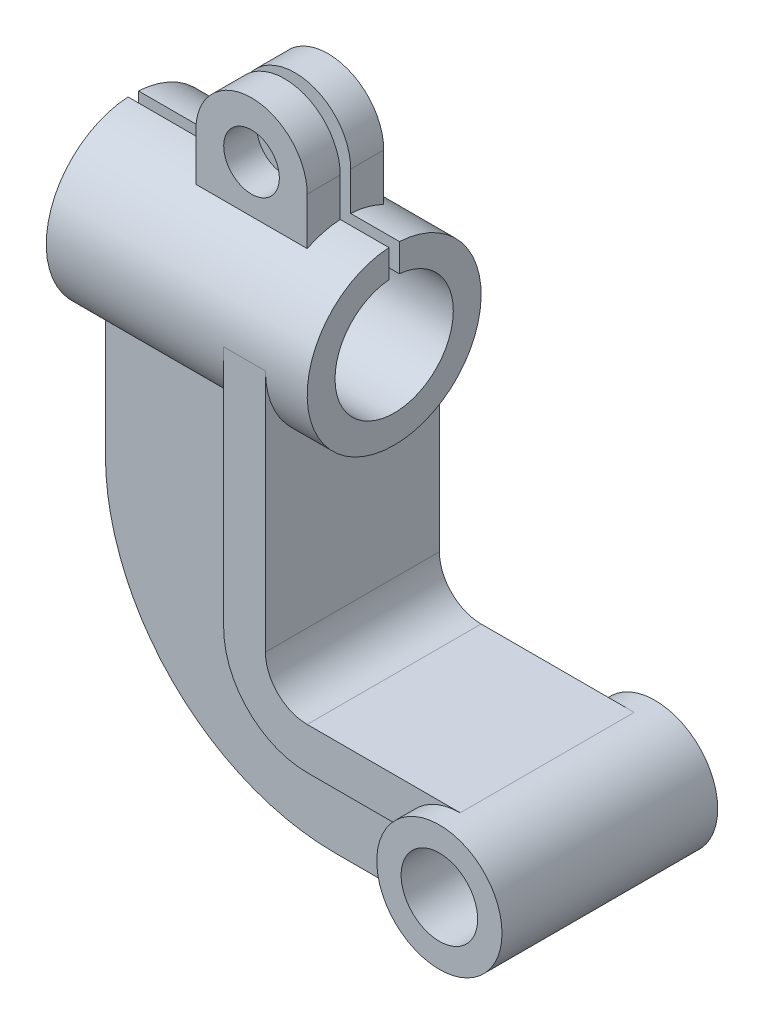
ISO-10303-21;
HEADER;
FILE_DESCRIPTION(('STEP AP214'),'2;1');
FILE_NAME('part.step','',(''),(''),'','','');
FILE_SCHEMA(('AUTOMOTIVE_DESIGN { 1 0 10303 214 1 1 1 1 }'));
ENDSEC;
DATA;
#1=APPLICATION_CONTEXT('core data for automotive mechanical design processes');
#2=APPLICATION_PROTOCOL_DEFINITION('international standard','automotive_design',2000,#1);
#3=PRODUCT_CONTEXT('',#1,'mechanical');
#4=PRODUCT('Part','Part','',(#3));
#5=PRODUCT_RELATED_PRODUCT_CATEGORY('part','',(#4));
#6=PRODUCT_DEFINITION_FORMATION('','',#4);
#7=PRODUCT_DEFINITION_CONTEXT('part definition',#1,'design');
#8=PRODUCT_DEFINITION('design','',#6,#7);
#9=PRODUCT_DEFINITION_SHAPE('','',#8);
#10=(LENGTH_UNIT() NAMED_UNIT(*) SI_UNIT(.MILLI.,.METRE.));
#11=(NAMED_UNIT(*) PLANE_ANGLE_UNIT() SI_UNIT($,.RADIAN.));
#12=(NAMED_UNIT(*) SI_UNIT($,.STERADIAN.) SOLID_ANGLE_UNIT());
#13=UNCERTAINTY_MEASURE_WITH_UNIT(LENGTH_MEASURE(1.E-05),#10,'distance_accuracy_value','');
#14=(GEOMETRIC_REPRESENTATION_CONTEXT(3) GLOBAL_UNCERTAINTY_ASSIGNED_CONTEXT((#13)) GLOBAL_UNIT_ASSIGNED_CONTEXT((#10,
#11,#12)) REPRESENTATION_CONTEXT('',''));
#15=CARTESIAN_POINT('',(0.,0.,0.));
#16=DIRECTION('',(0.,0.,1.));
#17=DIRECTION('',(1.,0.,0.));
#18=AXIS2_PLACEMENT_3D('',#15,#16,#17);
#19=CARTESIAN_POINT('',(-119.,100.,0.));
#20=DIRECTION('',(1.,0.,0.));
#21=DIRECTION('',(0.,0.,-1.));
#22=AXIS2_PLACEMENT_3D('',#19,#20,#21);
#23=CYLINDRICAL_SURFACE('',#22,17.);
#24=DIRECTION('',(1.,0.,0.));
#25=VECTOR('',#24,1.);
#26=CARTESIAN_POINT('',(-119.001,116.933694221876,-1.5));
#27=LINE('',#26,#25);
#28=CARTESIAN_POINT('',(-119.,116.933694221876,-1.5));
#29=VERTEX_POINT('',#28);
#30=CARTESIAN_POINT('',(-44.,116.933694221876,-1.5));
#31=VERTEX_POINT('',#30);
#32=EDGE_CURVE('E226',#29,#31,#27,.T.);
#33=ORIENTED_EDGE('',*,*,#32,.F.);
#34=CARTESIAN_POINT('',(-119.,100.,0.));
#35=DIRECTION('',(1.,0.,0.));
#36=DIRECTION('',(0.,0.,-1.));
#37=AXIS2_PLACEMENT_3D('',#34,#35,#36);
#38=CIRCLE('',#37,17.);
#39=CARTESIAN_POINT('',(-119.,116.933694221876,1.5));
#40=VERTEX_POINT('',#39);
#41=EDGE_CURVE('E243',#40,#29,#38,.T.);
#42=ORIENTED_EDGE('',*,*,#41,.F.);
#43=DIRECTION('',(1.,0.,0.));
#44=VECTOR('',#43,1.);
#45=CARTESIAN_POINT('',(-119.001,116.933694221876,1.5));
#46=LINE('',#45,#44);
#47=CARTESIAN_POINT('',(-44.,116.933694221876,1.5));
#48=VERTEX_POINT('',#47);
#49=EDGE_CURVE('E246',#40,#48,#46,.T.);
#50=ORIENTED_EDGE('',*,*,#49,.T.);
#51=CARTESIAN_POINT('',(-44.,100.,0.));
#52=DIRECTION('',(1.,0.,0.));
#53=DIRECTION('',(0.,0.,-1.));
#54=AXIS2_PLACEMENT_3D('',#51,#52,#53);
#55=CIRCLE('',#54,17.);
#56=EDGE_CURVE('E244',#48,#31,#55,.T.);
#57=ORIENTED_EDGE('',*,*,#56,.T.);
#58=EDGE_LOOP('',(#33,#42,#50,#57));
#59=FACE_BOUND('',#58,.T.);
#60=ADVANCED_FACE('F43',(#59),#23,.F.);
#61=CARTESIAN_POINT('',(-119.,0.,0.));
#62=DIRECTION('',(1.,0.,0.));
#63=DIRECTION('',(0.,0.,-1.));
#64=AXIS2_PLACEMENT_3D('',#61,#62,#63);
#65=PLANE('',#64);
#66=DIRECTION('',(0.,-1.,0.));
#67=VECTOR('',#66,1.);
#68=CARTESIAN_POINT('',(-119.,152.,-1.5));
#69=LINE('',#68,#67);
#70=CARTESIAN_POINT('',(-119.,124.954959426936,-1.5));
#71=VERTEX_POINT('',#70);
#72=EDGE_CURVE('E224',#71,#29,#69,.T.);
#73=ORIENTED_EDGE('',*,*,#72,.F.);
#74=CARTESIAN_POINT('',(-119.,100.,0.));
#75=DIRECTION('',(1.,0.,0.));
#76=DIRECTION('',(0.,0.,-1.));
#77=AXIS2_PLACEMENT_3D('',#74,#75,#76);
#78=CIRCLE('',#77,25.);
#79=CARTESIAN_POINT('',(-119.,124.954959426936,1.5));
#80=VERTEX_POINT('',#79);
#81=EDGE_CURVE('E252',#80,#71,#78,.T.);
#82=ORIENTED_EDGE('',*,*,#81,.F.);
#83=DIRECTION('',(0.,1.,0.));
#84=VECTOR('',#83,1.);
#85=CARTESIAN_POINT('',(-119.,152.,1.5));
#86=LINE('',#85,#84);
#87=EDGE_CURVE('E249',#40,#80,#86,.T.);
#88=ORIENTED_EDGE('',*,*,#87,.F.);
#89=ORIENTED_EDGE('',*,*,#41,.T.);
#90=EDGE_LOOP('',(#73,#82,#88,#89));
#91=FACE_BOUND('',#90,.T.);
#92=ADVANCED_FACE('F248',(#91),#65,.F.);
#93=CARTESIAN_POINT('',(-90.,136.,11.));
#94=DIRECTION('',(1.,0.,0.));
#95=DIRECTION('',(0.,0.,-1.));
#96=AXIS2_PLACEMENT_3D('',#93,#94,#95);
#97=PLANE('',#96);
#98=CARTESIAN_POINT('',(-90.,100.,0.));
#99=DIRECTION('',(1.,0.,0.));
#100=DIRECTION('',(0.,0.,-1.));
#101=AXIS2_PLACEMENT_3D('',#98,#99,#100);
#102=CIRCLE('',#101,25.);
#103=CARTESIAN_POINT('',(-90.,124.954959426936,-1.5));
#104=VERTEX_POINT('',#103);
#105=CARTESIAN_POINT('',(-90.,122.449944320644,-11.));
#106=VERTEX_POINT('',#105);
#107=EDGE_CURVE('E49',#104,#106,#102,.F.);
#108=ORIENTED_EDGE('',*,*,#107,.F.);
#109=DIRECTION('',(0.,-1.,0.));
#110=VECTOR('',#109,1.);
#111=CARTESIAN_POINT('',(-90.,152.,-1.5));
#112=LINE('',#111,#110);
#113=CARTESIAN_POINT('',(-90.,136.,-1.5));
#114=VERTEX_POINT('',#113);
#115=EDGE_CURVE('E240',#114,#104,#112,.T.);
#116=ORIENTED_EDGE('',*,*,#115,.F.);
#117=DIRECTION('',(0.,0.,-1.));
#118=VECTOR('',#117,1.);
#119=CARTESIAN_POINT('',(-90.,136.,11.));
#120=LINE('',#119,#118);
#121=CARTESIAN_POINT('',(-90.,136.,-11.));
#122=VERTEX_POINT('',#121);
#123=EDGE_CURVE('E301',#114,#122,#120,.T.);
#124=ORIENTED_EDGE('',*,*,#123,.T.);
#125=DIRECTION('',(0.,-1.,0.));
#126=VECTOR('',#125,1.);
#127=CARTESIAN_POINT('',(-90.,136.,-11.));
#128=LINE('',#127,#126);
#129=EDGE_CURVE('E298',#122,#106,#128,.T.);
#130=ORIENTED_EDGE('',*,*,#129,.T.);
#131=EDGE_LOOP('',(#108,#116,#124,#130));
#132=FACE_BOUND('',#131,.T.);
#133=ADVANCED_FACE('F299',(#132),#97,.F.);
#134=CARTESIAN_POINT('',(-58.,136.,11.));
#135=DIRECTION('',(-1.,0.,0.));
#136=DIRECTION('',(0.,-1.,0.));
#137=AXIS2_PLACEMENT_3D('',#134,#135,#136);
#138=PLANE('',#137);
#139=DIRECTION('',(0.,0.,-1.));
#140=VECTOR('',#139,1.);
#141=CARTESIAN_POINT('',(-58.,136.,11.));
#142=LINE('',#141,#140);
#143=CARTESIAN_POINT('',(-58.,136.,-1.5));
#144=VERTEX_POINT('',#143);
#145=CARTESIAN_POINT('',(-58.,136.,-11.));
#146=VERTEX_POINT('',#145);
#147=EDGE_CURVE('E316',#144,#146,#142,.T.);
#148=ORIENTED_EDGE('',*,*,#147,.F.);
#149=DIRECTION('',(0.,1.,0.));
#150=VECTOR('',#149,1.);
#151=CARTESIAN_POINT('',(-58.,152.,-1.5));
#152=LINE('',#151,#150);
#153=CARTESIAN_POINT('',(-58.,124.954959426936,-1.5));
#154=VERTEX_POINT('',#153);
#155=EDGE_CURVE('E756',#154,#144,#152,.T.);
#156=ORIENTED_EDGE('',*,*,#155,.F.);
#157=CARTESIAN_POINT('',(-58.,100.,0.));
#158=DIRECTION('',(-1.,0.,0.));
#159=DIRECTION('',(0.,-1.,0.));
#160=AXIS2_PLACEMENT_3D('',#157,#158,#159);
#161=CIRCLE('',#160,25.);
#162=CARTESIAN_POINT('',(-58.,122.449944320644,-11.));
#163=VERTEX_POINT('',#162);
#164=EDGE_CURVE('E275',#163,#154,#161,.F.);
#165=ORIENTED_EDGE('',*,*,#164,.F.);
#166=DIRECTION('',(0.,1.,0.));
#167=VECTOR('',#166,1.);
#168=CARTESIAN_POINT('',(-58.,136.,-11.));
#169=LINE('',#168,#167);
#170=EDGE_CURVE('E296',#163,#146,#169,.T.);
#171=ORIENTED_EDGE('',*,*,#170,.T.);
#172=EDGE_LOOP('',(#148,#156,#165,#171));
#173=FACE_BOUND('',#172,.T.);
#174=ADVANCED_FACE('F529',(#173),#138,.F.);
#175=CARTESIAN_POINT('',(-74.,136.,11.));
#176=DIRECTION('',(0.,0.,-1.));
#177=DIRECTION('',(-1.,0.,0.));
#178=AXIS2_PLACEMENT_3D('',#175,#176,#177);
#179=CYLINDRICAL_SURFACE('',#178,16.);
#180=CARTESIAN_POINT('',(-74.,136.,1.5));
#181=DIRECTION('',(0.,0.,1.));
#182=DIRECTION('',(0.,-1.,0.));
#183=AXIS2_PLACEMENT_3D('',#180,#181,#182);
#184=CIRCLE('',#183,16.);
#185=CARTESIAN_POINT('',(-90.,136.,1.5));
#186=VERTEX_POINT('',#185);
#187=CARTESIAN_POINT('',(-58.,136.,1.5));
#188=VERTEX_POINT('',#187);
#189=EDGE_CURVE('E63',#186,#188,#184,.F.);
#190=ORIENTED_EDGE('',*,*,#189,.F.);
#191=CARTESIAN_POINT('',(-90.,136.,11.));
#192=VERTEX_POINT('',#191);
#193=EDGE_CURVE('E317',#192,#186,#120,.T.);
#194=ORIENTED_EDGE('',*,*,#193,.F.);
#195=CARTESIAN_POINT('',(-74.,136.,11.));
#196=DIRECTION('',(0.,0.,1.));
#197=DIRECTION('',(1.,0.,0.));
#198=AXIS2_PLACEMENT_3D('',#195,#196,#197);
#199=CIRCLE('',#198,16.);
#200=CARTESIAN_POINT('',(-58.,136.,11.));
#201=VERTEX_POINT('',#200);
#202=EDGE_CURVE('E311',#201,#192,#199,.T.);
#203=ORIENTED_EDGE('',*,*,#202,.F.);
#204=EDGE_CURVE('E318',#201,#188,#142,.T.);
#205=ORIENTED_EDGE('',*,*,#204,.T.);
#206=EDGE_LOOP('',(#190,#194,#203,#205));
#207=FACE_BOUND('',#206,.T.);
#208=ADVANCED_FACE('F551',(#207),#179,.T.);
#209=CARTESIAN_POINT('',(-74.,136.,-1.5));
#210=DIRECTION('',(0.,0.,-1.));
#211=DIRECTION('',(0.,1.,0.));
#212=AXIS2_PLACEMENT_3D('',#209,#210,#211);
#213=CIRCLE('',#212,16.);
#214=EDGE_CURVE('E754',#144,#114,#213,.F.);
#215=ORIENTED_EDGE('',*,*,#214,.F.);
#216=ORIENTED_EDGE('',*,*,#147,.T.);
#217=CARTESIAN_POINT('',(-74.,136.,-11.));
#218=DIRECTION('',(0.,0.,1.));
#219=DIRECTION('',(1.,0.,0.));
#220=AXIS2_PLACEMENT_3D('',#217,#218,#219);
#221=CIRCLE('',#220,16.);
#222=EDGE_CURVE('E304',#146,#122,#221,.T.);
#223=ORIENTED_EDGE('',*,*,#222,.T.);
#224=ORIENTED_EDGE('',*,*,#123,.F.);
#225=EDGE_LOOP('',(#215,#216,#223,#224));
#226=FACE_BOUND('',#225,.T.);
#227=ADVANCED_FACE('F548',(#226),#179,.T.);
#228=CARTESIAN_POINT('',(-74.,136.,11.));
#229=DIRECTION('',(0.,0.,-1.));
#230=DIRECTION('',(-1.,0.,0.));
#231=AXIS2_PLACEMENT_3D('',#228,#229,#230);
#232=CYLINDRICAL_SURFACE('',#231,8.);
#233=CARTESIAN_POINT('',(-74.,136.,-1.5));
#234=DIRECTION('',(0.,0.,-1.));
#235=DIRECTION('',(0.,1.,0.));
#236=AXIS2_PLACEMENT_3D('',#233,#234,#235);
#237=CIRCLE('',#236,8.);
#238=CARTESIAN_POINT('',(-74.,144.,-1.5));
#239=VERTEX_POINT('',#238);
#240=EDGE_CURVE('E751',#239,#239,#237,.F.);
#241=ORIENTED_EDGE('',*,*,#240,.T.);
#242=EDGE_LOOP('',(#241));
#243=FACE_BOUND('',#242,.T.);
#244=CARTESIAN_POINT('',(-74.,136.,-11.));
#245=DIRECTION('',(0.,0.,1.));
#246=DIRECTION('',(1.,0.,0.));
#247=AXIS2_PLACEMENT_3D('',#244,#245,#246);
#248=CIRCLE('',#247,8.);
#249=CARTESIAN_POINT('',(-66.,136.,-11.));
#250=VERTEX_POINT('',#249);
#251=EDGE_CURVE('E308',#250,#250,#248,.T.);
#252=ORIENTED_EDGE('',*,*,#251,.F.);
#253=EDGE_LOOP('',(#252));
#254=FACE_BOUND('',#253,.T.);
#255=ADVANCED_FACE('F538',(#243,#254),#232,.F.);
#256=CARTESIAN_POINT('',(-119.,100.,0.));
#257=DIRECTION('',(1.,0.,0.));
#258=DIRECTION('',(0.,0.,-1.));
#259=AXIS2_PLACEMENT_3D('',#256,#257,#258);
#260=CYLINDRICAL_SURFACE('',#259,25.);
#261=DIRECTION('',(1.,0.,0.));
#262=VECTOR('',#261,1.);
#263=CARTESIAN_POINT('',(-119.,124.954959426936,-1.5));
#264=LINE('',#263,#262);
#265=CARTESIAN_POINT('',(-44.,124.954959426936,-1.5));
#266=VERTEX_POINT('',#265);
#267=EDGE_CURVE('E60',#154,#266,#264,.T.);
#268=ORIENTED_EDGE('',*,*,#267,.T.);
#269=CARTESIAN_POINT('',(-44.,100.,0.));
#270=DIRECTION('',(1.,0.,0.));
#271=DIRECTION('',(0.,0.,-1.));
#272=AXIS2_PLACEMENT_3D('',#269,#270,#271);
#273=CIRCLE('',#272,25.);
#274=CARTESIAN_POINT('',(-44.,124.954959426936,1.5));
#275=VERTEX_POINT('',#274);
#276=EDGE_CURVE('E255',#275,#266,#273,.T.);
#277=ORIENTED_EDGE('',*,*,#276,.F.);
#278=DIRECTION('',(1.,0.,0.));
#279=VECTOR('',#278,1.);
#280=CARTESIAN_POINT('',(-119.,124.954959426936,1.5));
#281=LINE('',#280,#279);
#282=CARTESIAN_POINT('',(-58.,124.954959426936,1.5));
#283=VERTEX_POINT('',#282);
#284=EDGE_CURVE('E786',#275,#283,#281,.F.);
#285=ORIENTED_EDGE('',*,*,#284,.T.);
#286=CARTESIAN_POINT('',(-58.,122.449944320644,11.));
#287=VERTEX_POINT('',#286);
#288=EDGE_CURVE('E272',#283,#287,#161,.F.);
#289=ORIENTED_EDGE('',*,*,#288,.T.);
#290=DIRECTION('',(1.,0.,0.));
#291=VECTOR('',#290,1.);
#292=CARTESIAN_POINT('',(-119.,122.449944320644,11.));
#293=LINE('',#292,#291);
#294=CARTESIAN_POINT('',(-90.,122.449944320644,11.));
#295=VERTEX_POINT('',#294);
#296=EDGE_CURVE('E280',#295,#287,#293,.T.);
#297=ORIENTED_EDGE('',*,*,#296,.F.);
#298=CARTESIAN_POINT('',(-90.,124.954959426936,1.5));
#299=VERTEX_POINT('',#298);
#300=EDGE_CURVE('E11',#295,#299,#102,.F.);
#301=ORIENTED_EDGE('',*,*,#300,.T.);
#302=EDGE_CURVE('E782',#299,#80,#281,.F.);
#303=ORIENTED_EDGE('',*,*,#302,.T.);
#304=ORIENTED_EDGE('',*,*,#81,.T.);
#305=EDGE_CURVE('E233',#71,#104,#264,.T.);
#306=ORIENTED_EDGE('',*,*,#305,.T.);
#307=ORIENTED_EDGE('',*,*,#107,.T.);
#308=DIRECTION('',(1.,0.,0.));
#309=VECTOR('',#308,1.);
#310=CARTESIAN_POINT('',(-119.,122.449944320644,-11.));
#311=LINE('',#310,#309);
#312=EDGE_CURVE('E273',#106,#163,#311,.T.);
#313=ORIENTED_EDGE('',*,*,#312,.T.);
#314=ORIENTED_EDGE('',*,*,#164,.T.);
#315=EDGE_LOOP('',(#268,#277,#285,#289,#297,#301,#303,#304,#306,#307,#313,#314));
#316=FACE_BOUND('',#315,.T.);
#317=CARTESIAN_POINT('',(-110.,100.,0.));
#318=DIRECTION('',(1.,0.,0.));
#319=DIRECTION('',(0.,0.,-1.));
#320=AXIS2_PLACEMENT_3D('',#317,#318,#319);
#321=CIRCLE('',#320,25.);
#322=CARTESIAN_POINT('',(-110.,81.6696972201766,-17.));
#323=VERTEX_POINT('',#322);
#324=CARTESIAN_POINT('',(-110.,81.6696972201766,17.));
#325=VERTEX_POINT('',#324);
#326=EDGE_CURVE('E266',#323,#325,#321,.F.);
#327=ORIENTED_EDGE('',*,*,#326,.T.);
#328=DIRECTION('',(1.,0.,0.));
#329=VECTOR('',#328,1.);
#330=CARTESIAN_POINT('',(-119.,81.6696972201766,17.));
#331=LINE('',#330,#329);
#332=CARTESIAN_POINT('',(-68.,81.6696972201766,17.));
#333=VERTEX_POINT('',#332);
#334=EDGE_CURVE('E378',#325,#333,#331,.T.);
#335=ORIENTED_EDGE('',*,*,#334,.T.);
#336=CARTESIAN_POINT('',(-68.,100.,0.));
#337=DIRECTION('',(1.,0.,0.));
#338=DIRECTION('',(0.,0.,-1.));
#339=AXIS2_PLACEMENT_3D('',#336,#337,#338);
#340=CIRCLE('',#339,25.);
#341=CARTESIAN_POINT('',(-68.,100.,25.));
#342=VERTEX_POINT('',#341);
#343=EDGE_CURVE('E251',#333,#342,#340,.F.);
#344=ORIENTED_EDGE('',*,*,#343,.T.);
#345=DIRECTION('',(-1.,0.,0.));
#346=VECTOR('',#345,1.);
#347=CARTESIAN_POINT('',(-68.,100.,25.));
#348=LINE('',#347,#346);
#349=CARTESIAN_POINT('',(-56.,100.,25.));
#350=VERTEX_POINT('',#349);
#351=EDGE_CURVE('E392',#350,#342,#348,.T.);
#352=ORIENTED_EDGE('',*,*,#351,.F.);
#353=CARTESIAN_POINT('',(-56.,100.,0.));
#354=DIRECTION('',(-1.,0.,0.));
#355=DIRECTION('',(0.,-1.,0.));
#356=AXIS2_PLACEMENT_3D('',#353,#354,#355);
#357=CIRCLE('',#356,25.);
#358=CARTESIAN_POINT('',(-56.,100.,-25.));
#359=VERTEX_POINT('',#358);
#360=EDGE_CURVE('E268',#350,#359,#357,.F.);
#361=ORIENTED_EDGE('',*,*,#360,.T.);
#362=DIRECTION('',(-1.,0.,0.));
#363=VECTOR('',#362,1.);
#364=CARTESIAN_POINT('',(-68.,100.,-25.));
#365=LINE('',#364,#363);
#366=CARTESIAN_POINT('',(-68.,100.,-25.));
#367=VERTEX_POINT('',#366);
#368=EDGE_CURVE('E418',#359,#367,#365,.T.);
#369=ORIENTED_EDGE('',*,*,#368,.T.);
#370=CARTESIAN_POINT('',(-68.,81.6696972201766,-17.));
#371=VERTEX_POINT('',#370);
#372=EDGE_CURVE('E263',#367,#371,#340,.F.);
#373=ORIENTED_EDGE('',*,*,#372,.T.);
#374=DIRECTION('',(1.,0.,0.));
#375=VECTOR('',#374,1.);
#376=CARTESIAN_POINT('',(-119.,81.6696972201766,-17.));
#377=LINE('',#376,#375);
#378=EDGE_CURVE('E371',#323,#371,#377,.T.);
#379=ORIENTED_EDGE('',*,*,#378,.F.);
#380=EDGE_LOOP('',(#327,#335,#344,#352,#361,#369,#373,#379));
#381=FACE_BOUND('',#380,.T.);
#382=ADVANCED_FACE('F284',(#316,#381),#260,.T.);
#383=CARTESIAN_POINT('',(-16.9705627484771,6.,25.));
#384=DIRECTION('',(0.,1.,0.));
#385=DIRECTION('',(0.,0.,1.));
#386=AXIS2_PLACEMENT_3D('',#383,#384,#385);
#387=PLANE('',#386);
#388=DIRECTION('',(-1.,0.,0.));
#389=VECTOR('',#388,1.);
#390=CARTESIAN_POINT('',(-16.9705627484771,6.,17.));
#391=LINE('',#390,#389);
#392=CARTESIAN_POINT('',(-16.9705627484771,6.,17.));
#393=VERTEX_POINT('',#392);
#394=CARTESIAN_POINT('',(-43.9999999999999,6.,17.));
#395=VERTEX_POINT('',#394);
#396=EDGE_CURVE('E380',#393,#395,#391,.T.);
#397=ORIENTED_EDGE('',*,*,#396,.F.);
#398=DIRECTION('',(0.,0.,-1.));
#399=VECTOR('',#398,1.);
#400=CARTESIAN_POINT('',(-16.9705627484771,6.,25.));
#401=LINE('',#400,#399);
#402=CARTESIAN_POINT('',(-16.9705627484771,6.,25.));
#403=VERTEX_POINT('',#402);
#404=EDGE_CURVE('E430',#403,#393,#401,.T.);
#405=ORIENTED_EDGE('',*,*,#404,.F.);
#406=DIRECTION('',(1.,0.,0.));
#407=VECTOR('',#406,1.);
#408=CARTESIAN_POINT('',(-16.9705627484771,6.,25.));
#409=LINE('',#408,#407);
#410=CARTESIAN_POINT('',(-43.9999999999999,6.,25.));
#411=VERTEX_POINT('',#410);
#412=EDGE_CURVE('E402',#411,#403,#409,.T.);
#413=ORIENTED_EDGE('',*,*,#412,.F.);
#414=DIRECTION('',(0.,0.,-1.));
#415=VECTOR('',#414,1.);
#416=CARTESIAN_POINT('',(-43.9999999999999,6.,25.));
#417=LINE('',#416,#415);
#418=EDGE_CURVE('E427',#411,#395,#417,.T.);
#419=ORIENTED_EDGE('',*,*,#418,.T.);
#420=EDGE_LOOP('',(#397,#405,#413,#419));
#421=FACE_BOUND('',#420,.T.);
#422=ADVANCED_FACE('F477',(#421),#387,.F.);
#423=CARTESIAN_POINT('',(-44.,30.,25.));
#424=DIRECTION('',(0.,0.,-1.));
#425=DIRECTION('',(-1.,0.,0.));
#426=AXIS2_PLACEMENT_3D('',#423,#424,#425);
#427=CYLINDRICAL_SURFACE('',#426,24.);
#428=CARTESIAN_POINT('',(-44.,30.,17.));
#429=DIRECTION('',(0.,0.,-1.));
#430=DIRECTION('',(-1.,0.,0.));
#431=AXIS2_PLACEMENT_3D('',#428,#429,#430);
#432=CIRCLE('',#431,24.);
#433=CARTESIAN_POINT('',(-68.,30.0000000000002,17.));
#434=VERTEX_POINT('',#433);
#435=EDGE_CURVE('E374',#395,#434,#432,.T.);
#436=ORIENTED_EDGE('',*,*,#435,.F.);
#437=ORIENTED_EDGE('',*,*,#418,.F.);
#438=CARTESIAN_POINT('',(-44.,30.,25.));
#439=DIRECTION('',(0.,0.,1.));
#440=DIRECTION('',(1.,0.,0.));
#441=AXIS2_PLACEMENT_3D('',#438,#439,#440);
#442=CIRCLE('',#441,24.);
#443=CARTESIAN_POINT('',(-68.,30.0000000000002,25.));
#444=VERTEX_POINT('',#443);
#445=EDGE_CURVE('E397',#444,#411,#442,.T.);
#446=ORIENTED_EDGE('',*,*,#445,.F.);
#447=DIRECTION('',(0.,0.,-1.));
#448=VECTOR('',#447,1.);
#449=CARTESIAN_POINT('',(-68.,30.0000000000002,25.));
#450=LINE('',#449,#448);
#451=EDGE_CURVE('E432',#444,#434,#450,.T.);
#452=ORIENTED_EDGE('',*,*,#451,.T.);
#453=EDGE_LOOP('',(#436,#437,#446,#452));
#454=FACE_BOUND('',#453,.T.);
#455=ADVANCED_FACE('F476',(#454),#427,.T.);
#456=CARTESIAN_POINT('',(-68.,30.0000000000002,25.));
#457=DIRECTION('',(1.,0.,0.));
#458=DIRECTION('',(0.,0.,-1.));
#459=AXIS2_PLACEMENT_3D('',#456,#457,#458);
#460=PLANE('',#459);
#461=DIRECTION('',(0.,1.,0.));
#462=VECTOR('',#461,1.);
#463=CARTESIAN_POINT('',(-68.,30.0000000000002,17.));
#464=LINE('',#463,#462);
#465=EDGE_CURVE('E373',#434,#333,#464,.T.);
#466=ORIENTED_EDGE('',*,*,#465,.F.);
#467=ORIENTED_EDGE('',*,*,#451,.F.);
#468=DIRECTION('',(0.,-1.,0.));
#469=VECTOR('',#468,1.);
#470=CARTESIAN_POINT('',(-68.,30.0000000000002,25.));
#471=LINE('',#470,#469);
#472=EDGE_CURVE('E400',#342,#444,#471,.T.);
#473=ORIENTED_EDGE('',*,*,#472,.F.);
#474=ORIENTED_EDGE('',*,*,#343,.F.);
#475=EDGE_LOOP('',(#466,#467,#473,#474));
#476=FACE_BOUND('',#475,.T.);
#477=ADVANCED_FACE('F466',(#476),#460,.F.);
#478=CARTESIAN_POINT('',(-44.,0.,0.));
#479=DIRECTION('',(1.,0.,0.));
#480=DIRECTION('',(0.,0.,-1.));
#481=AXIS2_PLACEMENT_3D('',#478,#479,#480);
#482=PLANE('',#481);
#483=DIRECTION('',(0.,1.,0.));
#484=VECTOR('',#483,1.);
#485=CARTESIAN_POINT('',(-44.,152.,-1.5));
#486=LINE('',#485,#484);
#487=EDGE_CURVE('E764',#31,#266,#486,.T.);
#488=ORIENTED_EDGE('',*,*,#487,.F.);
#489=ORIENTED_EDGE('',*,*,#56,.F.);
#490=DIRECTION('',(0.,-1.,0.));
#491=VECTOR('',#490,1.);
#492=CARTESIAN_POINT('',(-44.,152.,1.5));
#493=LINE('',#492,#491);
#494=EDGE_CURVE('E236',#275,#48,#493,.T.);
#495=ORIENTED_EDGE('',*,*,#494,.F.);
#496=ORIENTED_EDGE('',*,*,#276,.T.);
#497=EDGE_LOOP('',(#488,#489,#495,#496));
#498=FACE_BOUND('',#497,.T.);
#499=ADVANCED_FACE('F537',(#498),#482,.T.);
#500=CARTESIAN_POINT('',(0.,0.,-25.));
#501=DIRECTION('',(0.,0.,1.));
#502=DIRECTION('',(1.,0.,0.));
#503=AXIS2_PLACEMENT_3D('',#500,#501,#502);
#504=PLANE('',#503);
#505=CARTESIAN_POINT('',(0.,0.,-25.));
#506=DIRECTION('',(0.,0.,-1.));
#507=DIRECTION('',(1.,0.,0.));
#508=AXIS2_PLACEMENT_3D('',#505,#506,#507);
#509=CIRCLE('',#508,18.);
#510=CARTESIAN_POINT('',(-16.9705627484771,6.,-25.));
#511=VERTEX_POINT('',#510);
#512=CARTESIAN_POINT('',(0.,18.,-25.));
#513=VERTEX_POINT('',#512);
#514=EDGE_CURVE('E385',#511,#513,#509,.T.);
#515=ORIENTED_EDGE('',*,*,#514,.F.);
#516=DIRECTION('',(1.,0.,0.));
#517=VECTOR('',#516,1.);
#518=CARTESIAN_POINT('',(-16.9705627484771,6.,-25.));
#519=LINE('',#518,#517);
#520=CARTESIAN_POINT('',(-43.9999999999999,6.,-25.));
#521=VERTEX_POINT('',#520);
#522=EDGE_CURVE('E390',#521,#511,#519,.T.);
#523=ORIENTED_EDGE('',*,*,#522,.F.);
#524=CARTESIAN_POINT('',(-44.,30.,-25.));
#525=DIRECTION('',(0.,0.,1.));
#526=DIRECTION('',(1.,0.,0.));
#527=AXIS2_PLACEMENT_3D('',#524,#525,#526);
#528=CIRCLE('',#527,24.);
#529=CARTESIAN_POINT('',(-68.,30.0000000000002,-25.));
#530=VERTEX_POINT('',#529);
#531=EDGE_CURVE('E422',#530,#521,#528,.T.);
#532=ORIENTED_EDGE('',*,*,#531,.F.);
#533=DIRECTION('',(0.,-1.,0.));
#534=VECTOR('',#533,1.);
#535=CARTESIAN_POINT('',(-68.,30.0000000000002,-25.));
#536=LINE('',#535,#534);
#537=EDGE_CURVE('E417',#367,#530,#536,.T.);
#538=ORIENTED_EDGE('',*,*,#537,.F.);
#539=ORIENTED_EDGE('',*,*,#368,.F.);
#540=DIRECTION('',(0.,1.,0.));
#541=VECTOR('',#540,1.);
#542=CARTESIAN_POINT('',(-56.,30.0000000000001,-25.));
#543=LINE('',#542,#541);
#544=CARTESIAN_POINT('',(-56.,30.0000000000001,-25.));
#545=VERTEX_POINT('',#544);
#546=EDGE_CURVE('E413',#545,#359,#543,.T.);
#547=ORIENTED_EDGE('',*,*,#546,.F.);
#548=CARTESIAN_POINT('',(-44.,30.,-25.));
#549=DIRECTION('',(0.,0.,-1.));
#550=DIRECTION('',(1.,0.,0.));
#551=AXIS2_PLACEMENT_3D('',#548,#549,#550);
#552=CIRCLE('',#551,12.);
#553=CARTESIAN_POINT('',(-43.9999999999999,18.,-25.));
#554=VERTEX_POINT('',#553);
#555=EDGE_CURVE('E408',#554,#545,#552,.T.);
#556=ORIENTED_EDGE('',*,*,#555,.F.);
#557=DIRECTION('',(-1.,0.,0.));
#558=VECTOR('',#557,1.);
#559=CARTESIAN_POINT('',(0.,18.,-25.));
#560=LINE('',#559,#558);
#561=EDGE_CURVE('E410',#513,#554,#560,.T.);
#562=ORIENTED_EDGE('',*,*,#561,.F.);
#563=EDGE_LOOP('',(#515,#523,#532,#538,#539,#547,#556,#562));
#564=FACE_BOUND('',#563,.T.);
#565=ADVANCED_FACE('F454',(#564),#504,.F.);
#566=CARTESIAN_POINT('',(0.,0.,25.));
#567=DIRECTION('',(0.,0.,1.));
#568=DIRECTION('',(1.,0.,0.));
#569=AXIS2_PLACEMENT_3D('',#566,#567,#568);
#570=PLANE('',#569);
#571=CARTESIAN_POINT('',(0.,0.,25.));
#572=DIRECTION('',(0.,0.,-1.));
#573=DIRECTION('',(1.,0.,0.));
#574=AXIS2_PLACEMENT_3D('',#571,#572,#573);
#575=CIRCLE('',#574,18.);
#576=CARTESIAN_POINT('',(0.,18.,25.));
#577=VERTEX_POINT('',#576);
#578=EDGE_CURVE('E384',#403,#577,#575,.T.);
#579=ORIENTED_EDGE('',*,*,#578,.T.);
#580=DIRECTION('',(-1.,0.,0.));
#581=VECTOR('',#580,1.);
#582=CARTESIAN_POINT('',(0.,18.,25.));
#583=LINE('',#582,#581);
#584=CARTESIAN_POINT('',(-43.9999999999999,18.,25.));
#585=VERTEX_POINT('',#584);
#586=EDGE_CURVE('E387',#577,#585,#583,.T.);
#587=ORIENTED_EDGE('',*,*,#586,.T.);
#588=CARTESIAN_POINT('',(-44.,30.,25.));
#589=DIRECTION('',(0.,0.,-1.));
#590=DIRECTION('',(1.,0.,0.));
#591=AXIS2_PLACEMENT_3D('',#588,#589,#590);
#592=CIRCLE('',#591,12.);
#593=CARTESIAN_POINT('',(-56.,30.0000000000001,25.));
#594=VERTEX_POINT('',#593);
#595=EDGE_CURVE('E386',#585,#594,#592,.T.);
#596=ORIENTED_EDGE('',*,*,#595,.T.);
#597=DIRECTION('',(0.,1.,0.));
#598=VECTOR('',#597,1.);
#599=CARTESIAN_POINT('',(-56.,30.0000000000001,25.));
#600=LINE('',#599,#598);
#601=EDGE_CURVE('E391',#594,#350,#600,.T.);
#602=ORIENTED_EDGE('',*,*,#601,.T.);
#603=ORIENTED_EDGE('',*,*,#351,.T.);
#604=ORIENTED_EDGE('',*,*,#472,.T.);
#605=ORIENTED_EDGE('',*,*,#445,.T.);
#606=ORIENTED_EDGE('',*,*,#412,.T.);
#607=EDGE_LOOP('',(#579,#587,#596,#602,#603,#604,#605,#606));
#608=FACE_BOUND('',#607,.T.);
#609=ADVANCED_FACE('F461',(#608),#570,.T.);
#610=CARTESIAN_POINT('',(-16.9705627484771,6.,-17.));
#611=VERTEX_POINT('',#610);
#612=EDGE_CURVE('E404',#611,#511,#401,.T.);
#613=ORIENTED_EDGE('',*,*,#612,.F.);
#614=DIRECTION('',(-1.,0.,0.));
#615=VECTOR('',#614,1.);
#616=CARTESIAN_POINT('',(-16.9705627484771,6.,-17.));
#617=LINE('',#616,#615);
#618=CARTESIAN_POINT('',(-43.9999999999999,6.,-17.));
#619=VERTEX_POINT('',#618);
#620=EDGE_CURVE('E368',#611,#619,#617,.T.);
#621=ORIENTED_EDGE('',*,*,#620,.T.);
#622=EDGE_CURVE('E429',#619,#521,#417,.T.);
#623=ORIENTED_EDGE('',*,*,#622,.T.);
#624=ORIENTED_EDGE('',*,*,#522,.T.);
#625=EDGE_LOOP('',(#613,#621,#623,#624));
#626=FACE_BOUND('',#625,.T.);
#627=ADVANCED_FACE('F491',(#626),#387,.F.);
#628=ORIENTED_EDGE('',*,*,#622,.F.);
#629=CARTESIAN_POINT('',(-44.,30.,-17.));
#630=DIRECTION('',(0.,0.,-1.));
#631=DIRECTION('',(-1.,0.,0.));
#632=AXIS2_PLACEMENT_3D('',#629,#630,#631);
#633=CIRCLE('',#632,24.);
#634=CARTESIAN_POINT('',(-68.,30.0000000000002,-17.));
#635=VERTEX_POINT('',#634);
#636=EDGE_CURVE('E362',#619,#635,#633,.T.);
#637=ORIENTED_EDGE('',*,*,#636,.T.);
#638=EDGE_CURVE('E433',#635,#530,#450,.T.);
#639=ORIENTED_EDGE('',*,*,#638,.T.);
#640=ORIENTED_EDGE('',*,*,#531,.T.);
#641=EDGE_LOOP('',(#628,#637,#639,#640));
#642=FACE_BOUND('',#641,.T.);
#643=ADVANCED_FACE('F498',(#642),#427,.T.);
#644=ORIENTED_EDGE('',*,*,#638,.F.);
#645=DIRECTION('',(0.,1.,0.));
#646=VECTOR('',#645,1.);
#647=CARTESIAN_POINT('',(-68.,30.0000000000002,-17.));
#648=LINE('',#647,#646);
#649=EDGE_CURVE('E359',#635,#371,#648,.T.);
#650=ORIENTED_EDGE('',*,*,#649,.T.);
#651=ORIENTED_EDGE('',*,*,#372,.F.);
#652=ORIENTED_EDGE('',*,*,#537,.T.);
#653=EDGE_LOOP('',(#644,#650,#651,#652));
#654=FACE_BOUND('',#653,.T.);
#655=ADVANCED_FACE('F501',(#654),#460,.F.);
#656=CARTESIAN_POINT('',(-56.,30.0000000000001,25.));
#657=DIRECTION('',(-1.,0.,0.));
#658=DIRECTION('',(0.,-1.,0.));
#659=AXIS2_PLACEMENT_3D('',#656,#657,#658);
#660=PLANE('',#659);
#661=ORIENTED_EDGE('',*,*,#546,.T.);
#662=ORIENTED_EDGE('',*,*,#360,.F.);
#663=ORIENTED_EDGE('',*,*,#601,.F.);
#664=DIRECTION('',(0.,0.,-1.));
#665=VECTOR('',#664,1.);
#666=CARTESIAN_POINT('',(-56.,30.0000000000001,25.));
#667=LINE('',#666,#665);
#668=EDGE_CURVE('E440',#594,#545,#667,.T.);
#669=ORIENTED_EDGE('',*,*,#668,.T.);
#670=EDGE_LOOP('',(#661,#662,#663,#669));
#671=FACE_BOUND('',#670,.T.);
#672=ADVANCED_FACE('F459',(#671),#660,.F.);
#673=CARTESIAN_POINT('',(-44.,30.,25.));
#674=DIRECTION('',(0.,0.,-1.));
#675=DIRECTION('',(-1.,0.,0.));
#676=AXIS2_PLACEMENT_3D('',#673,#674,#675);
#677=CYLINDRICAL_SURFACE('',#676,12.);
#678=ORIENTED_EDGE('',*,*,#555,.T.);
#679=ORIENTED_EDGE('',*,*,#668,.F.);
#680=ORIENTED_EDGE('',*,*,#595,.F.);
#681=DIRECTION('',(0.,0.,-1.));
#682=VECTOR('',#681,1.);
#683=CARTESIAN_POINT('',(-43.9999999999999,18.,25.));
#684=LINE('',#683,#682);
#685=EDGE_CURVE('E438',#585,#554,#684,.T.);
#686=ORIENTED_EDGE('',*,*,#685,.T.);
#687=EDGE_LOOP('',(#678,#679,#680,#686));
#688=FACE_BOUND('',#687,.T.);
#689=ADVANCED_FACE('F460',(#688),#677,.F.);
#690=CARTESIAN_POINT('',(0.,18.,25.));
#691=DIRECTION('',(0.,-1.,0.));
#692=DIRECTION('',(1.,0.,0.));
#693=AXIS2_PLACEMENT_3D('',#690,#691,#692);
#694=PLANE('',#693);
#695=ORIENTED_EDGE('',*,*,#561,.T.);
#696=ORIENTED_EDGE('',*,*,#685,.F.);
#697=ORIENTED_EDGE('',*,*,#586,.F.);
#698=DIRECTION('',(0.,0.,-1.));
#699=VECTOR('',#698,1.);
#700=CARTESIAN_POINT('',(0.,18.,25.));
#701=LINE('',#700,#699);
#702=EDGE_CURVE('E256',#577,#513,#701,.T.);
#703=ORIENTED_EDGE('',*,*,#702,.T.);
#704=EDGE_LOOP('',(#695,#696,#697,#703));
#705=FACE_BOUND('',#704,.T.);
#706=ADVANCED_FACE('F443',(#705),#694,.F.);
#707=CARTESIAN_POINT('',(0.,0.,31.));
#708=DIRECTION('',(0.,0.,-1.));
#709=DIRECTION('',(-1.,0.,0.));
#710=AXIS2_PLACEMENT_3D('',#707,#708,#709);
#711=CYLINDRICAL_SURFACE('',#710,18.);
#712=CARTESIAN_POINT('',(0.,0.,-31.));
#713=DIRECTION('',(0.,0.,1.));
#714=DIRECTION('',(1.,0.,0.));
#715=AXIS2_PLACEMENT_3D('',#712,#713,#714);
#716=CIRCLE('',#715,18.);
#717=CARTESIAN_POINT('',(18.,0.,-31.));
#718=VERTEX_POINT('',#717);
#719=EDGE_CURVE('E352',#718,#718,#716,.T.);
#720=ORIENTED_EDGE('',*,*,#719,.T.);
#721=EDGE_LOOP('',(#720));
#722=FACE_BOUND('',#721,.T.);
#723=CARTESIAN_POINT('',(0.,0.,31.));
#724=DIRECTION('',(0.,0.,1.));
#725=DIRECTION('',(1.,0.,0.));
#726=AXIS2_PLACEMENT_3D('',#723,#724,#725);
#727=CIRCLE('',#726,18.);
#728=CARTESIAN_POINT('',(18.,0.,31.));
#729=VERTEX_POINT('',#728);
#730=EDGE_CURVE('E357',#729,#729,#727,.T.);
#731=ORIENTED_EDGE('',*,*,#730,.F.);
#732=EDGE_LOOP('',(#731));
#733=FACE_BOUND('',#732,.T.);
#734=CARTESIAN_POINT('',(0.,0.,-17.));
#735=DIRECTION('',(0.,0.,-1.));
#736=DIRECTION('',(1.,0.,0.));
#737=AXIS2_PLACEMENT_3D('',#734,#735,#736);
#738=CIRCLE('',#737,18.);
#739=CARTESIAN_POINT('',(0.,-18.,-17.));
#740=VERTEX_POINT('',#739);
#741=EDGE_CURVE('E330',#740,#611,#738,.T.);
#742=ORIENTED_EDGE('',*,*,#741,.T.);
#743=ORIENTED_EDGE('',*,*,#612,.T.);
#744=ORIENTED_EDGE('',*,*,#514,.T.);
#745=ORIENTED_EDGE('',*,*,#702,.F.);
#746=ORIENTED_EDGE('',*,*,#578,.F.);
#747=ORIENTED_EDGE('',*,*,#404,.T.);
#748=CARTESIAN_POINT('',(0.,0.,17.));
#749=DIRECTION('',(0.,0.,-1.));
#750=DIRECTION('',(1.,0.,0.));
#751=AXIS2_PLACEMENT_3D('',#748,#749,#750);
#752=CIRCLE('',#751,18.);
#753=CARTESIAN_POINT('',(0.,-18.,17.));
#754=VERTEX_POINT('',#753);
#755=EDGE_CURVE('E333',#754,#393,#752,.T.);
#756=ORIENTED_EDGE('',*,*,#755,.F.);
#757=DIRECTION('',(0.,0.,-1.));
#758=VECTOR('',#757,1.);
#759=CARTESIAN_POINT('',(0.,-18.,17.));
#760=LINE('',#759,#758);
#761=EDGE_CURVE('E332',#754,#740,#760,.T.);
#762=ORIENTED_EDGE('',*,*,#761,.T.);
#763=EDGE_LOOP('',(#742,#743,#744,#745,#746,#747,#756,#762));
#764=FACE_BOUND('',#763,.T.);
#765=ADVANCED_FACE('F446',(#722,#733,#764),#711,.T.);
#766=CARTESIAN_POINT('',(0.,0.,31.));
#767=DIRECTION('',(0.,0.,1.));
#768=DIRECTION('',(1.,0.,0.));
#769=AXIS2_PLACEMENT_3D('',#766,#767,#768);
#770=PLANE('',#769);
#771=ORIENTED_EDGE('',*,*,#730,.T.);
#772=EDGE_LOOP('',(#771));
#773=FACE_BOUND('',#772,.T.);
#774=CARTESIAN_POINT('',(0.,0.,31.));
#775=DIRECTION('',(0.,0.,1.));
#776=DIRECTION('',(1.,0.,0.));
#777=AXIS2_PLACEMENT_3D('',#774,#775,#776);
#778=CIRCLE('',#777,11.);
#779=CARTESIAN_POINT('',(11.,0.,31.));
#780=VERTEX_POINT('',#779);
#781=EDGE_CURVE('E353',#780,#780,#778,.T.);
#782=ORIENTED_EDGE('',*,*,#781,.F.);
#783=EDGE_LOOP('',(#782));
#784=FACE_BOUND('',#783,.T.);
#785=ADVANCED_FACE('F810',(#773,#784),#770,.T.);
#786=CARTESIAN_POINT('',(0.,0.,-31.));
#787=DIRECTION('',(0.,0.,1.));
#788=DIRECTION('',(1.,0.,0.));
#789=AXIS2_PLACEMENT_3D('',#786,#787,#788);
#790=PLANE('',#789);
#791=ORIENTED_EDGE('',*,*,#719,.F.);
#792=EDGE_LOOP('',(#791));
#793=FACE_BOUND('',#792,.T.);
#794=CARTESIAN_POINT('',(0.,0.,-31.));
#795=DIRECTION('',(0.,0.,1.));
#796=DIRECTION('',(1.,0.,0.));
#797=AXIS2_PLACEMENT_3D('',#794,#795,#796);
#798=CIRCLE('',#797,11.);
#799=CARTESIAN_POINT('',(11.,0.,-31.));
#800=VERTEX_POINT('',#799);
#801=EDGE_CURVE('E349',#800,#800,#798,.T.);
#802=ORIENTED_EDGE('',*,*,#801,.T.);
#803=EDGE_LOOP('',(#802));
#804=FACE_BOUND('',#803,.T.);
#805=ADVANCED_FACE('F820',(#793,#804),#790,.F.);
#806=CARTESIAN_POINT('',(0.,0.,31.));
#807=DIRECTION('',(0.,0.,-1.));
#808=DIRECTION('',(-1.,0.,0.));
#809=AXIS2_PLACEMENT_3D('',#806,#807,#808);
#810=CYLINDRICAL_SURFACE('',#809,11.);
#811=ORIENTED_EDGE('',*,*,#781,.T.);
#812=EDGE_LOOP('',(#811));
#813=FACE_BOUND('',#812,.T.);
#814=ORIENTED_EDGE('',*,*,#801,.F.);
#815=EDGE_LOOP('',(#814));
#816=FACE_BOUND('',#815,.T.);
#817=ADVANCED_FACE('F516',(#813,#816),#810,.F.);
#818=CARTESIAN_POINT('',(-110.,88.5221019607843,17.));
#819=DIRECTION('',(1.,0.,0.));
#820=DIRECTION('',(0.,0.,-1.));
#821=AXIS2_PLACEMENT_3D('',#818,#819,#820);
#822=PLANE('',#821);
#823=ORIENTED_EDGE('',*,*,#326,.F.);
#824=DIRECTION('',(0.,-1.,0.));
#825=VECTOR('',#824,1.);
#826=CARTESIAN_POINT('',(-110.,88.5221019607843,-17.));
#827=LINE('',#826,#825);
#828=CARTESIAN_POINT('',(-110.,48.,-17.));
#829=VERTEX_POINT('',#828);
#830=EDGE_CURVE('E324',#323,#829,#827,.T.);
#831=ORIENTED_EDGE('',*,*,#830,.T.);
#832=DIRECTION('',(0.,0.,-1.));
#833=VECTOR('',#832,1.);
#834=CARTESIAN_POINT('',(-110.,48.,17.));
#835=LINE('',#834,#833);
#836=CARTESIAN_POINT('',(-110.,48.,17.));
#837=VERTEX_POINT('',#836);
#838=EDGE_CURVE('E350',#837,#829,#835,.T.);
#839=ORIENTED_EDGE('',*,*,#838,.F.);
#840=DIRECTION('',(0.,-1.,0.));
#841=VECTOR('',#840,1.);
#842=CARTESIAN_POINT('',(-110.,88.5221019607843,17.));
#843=LINE('',#842,#841);
#844=EDGE_CURVE('E321',#325,#837,#843,.T.);
#845=ORIENTED_EDGE('',*,*,#844,.F.);
#846=EDGE_LOOP('',(#823,#831,#839,#845));
#847=FACE_BOUND('',#846,.T.);
#848=ADVANCED_FACE('F507',(#847),#822,.F.);
#849=CARTESIAN_POINT('',(-44.,48.,17.));
#850=DIRECTION('',(0.,0.,-1.));
#851=DIRECTION('',(-1.,0.,0.));
#852=AXIS2_PLACEMENT_3D('',#849,#850,#851);
#853=CYLINDRICAL_SURFACE('',#852,66.);
#854=CARTESIAN_POINT('',(-44.,48.,-17.));
#855=DIRECTION('',(0.,0.,1.));
#856=DIRECTION('',(-1.,0.,0.));
#857=AXIS2_PLACEMENT_3D('',#854,#855,#856);
#858=CIRCLE('',#857,66.);
#859=CARTESIAN_POINT('',(-43.9999999999995,-18.,-17.));
#860=VERTEX_POINT('',#859);
#861=EDGE_CURVE('E337',#829,#860,#858,.T.);
#862=ORIENTED_EDGE('',*,*,#861,.T.);
#863=DIRECTION('',(0.,0.,-1.));
#864=VECTOR('',#863,1.);
#865=CARTESIAN_POINT('',(-43.9999999999995,-18.,17.));
#866=LINE('',#865,#864);
#867=CARTESIAN_POINT('',(-43.9999999999995,-18.,17.));
#868=VERTEX_POINT('',#867);
#869=EDGE_CURVE('E341',#868,#860,#866,.T.);
#870=ORIENTED_EDGE('',*,*,#869,.F.);
#871=CARTESIAN_POINT('',(-44.,48.,17.));
#872=DIRECTION('',(0.,0.,1.));
#873=DIRECTION('',(-1.,0.,0.));
#874=AXIS2_PLACEMENT_3D('',#871,#872,#873);
#875=CIRCLE('',#874,66.);
#876=EDGE_CURVE('E326',#837,#868,#875,.T.);
#877=ORIENTED_EDGE('',*,*,#876,.F.);
#878=ORIENTED_EDGE('',*,*,#838,.T.);
#879=EDGE_LOOP('',(#862,#870,#877,#878));
#880=FACE_BOUND('',#879,.T.);
#881=ADVANCED_FACE('F512',(#880),#853,.T.);
#882=CARTESIAN_POINT('',(-43.9999999999995,-18.,17.));
#883=DIRECTION('',(0.,1.,0.));
#884=DIRECTION('',(0.,0.,1.));
#885=AXIS2_PLACEMENT_3D('',#882,#883,#884);
#886=PLANE('',#885);
#887=DIRECTION('',(1.,0.,0.));
#888=VECTOR('',#887,1.);
#889=CARTESIAN_POINT('',(-43.9999999999995,-18.,-17.));
#890=LINE('',#889,#888);
#891=EDGE_CURVE('E336',#860,#740,#890,.T.);
#892=ORIENTED_EDGE('',*,*,#891,.T.);
#893=ORIENTED_EDGE('',*,*,#761,.F.);
#894=DIRECTION('',(1.,0.,0.));
#895=VECTOR('',#894,1.);
#896=CARTESIAN_POINT('',(-43.9999999999995,-18.,17.));
#897=LINE('',#896,#895);
#898=EDGE_CURVE('E327',#868,#754,#897,.T.);
#899=ORIENTED_EDGE('',*,*,#898,.F.);
#900=ORIENTED_EDGE('',*,*,#869,.T.);
#901=EDGE_LOOP('',(#892,#893,#899,#900));
#902=FACE_BOUND('',#901,.T.);
#903=ADVANCED_FACE('F486',(#902),#886,.F.);
#904=CARTESIAN_POINT('',(-44.,30.,17.));
#905=DIRECTION('',(0.,0.,-1.));
#906=DIRECTION('',(-1.,0.,0.));
#907=AXIS2_PLACEMENT_3D('',#904,#905,#906);
#908=PLANE('',#907);
#909=ORIENTED_EDGE('',*,*,#334,.F.);
#910=ORIENTED_EDGE('',*,*,#844,.T.);
#911=ORIENTED_EDGE('',*,*,#876,.T.);
#912=ORIENTED_EDGE('',*,*,#898,.T.);
#913=ORIENTED_EDGE('',*,*,#755,.T.);
#914=ORIENTED_EDGE('',*,*,#396,.T.);
#915=ORIENTED_EDGE('',*,*,#435,.T.);
#916=ORIENTED_EDGE('',*,*,#465,.T.);
#917=EDGE_LOOP('',(#909,#910,#911,#912,#913,#914,#915,#916));
#918=FACE_BOUND('',#917,.T.);
#919=ADVANCED_FACE('F485',(#918),#908,.F.);
#920=CARTESIAN_POINT('',(-44.,30.,-17.));
#921=DIRECTION('',(0.,0.,-1.));
#922=DIRECTION('',(-1.,0.,0.));
#923=AXIS2_PLACEMENT_3D('',#920,#921,#922);
#924=PLANE('',#923);
#925=ORIENTED_EDGE('',*,*,#830,.F.);
#926=ORIENTED_EDGE('',*,*,#378,.T.);
#927=ORIENTED_EDGE('',*,*,#649,.F.);
#928=ORIENTED_EDGE('',*,*,#636,.F.);
#929=ORIENTED_EDGE('',*,*,#620,.F.);
#930=ORIENTED_EDGE('',*,*,#741,.F.);
#931=ORIENTED_EDGE('',*,*,#891,.F.);
#932=ORIENTED_EDGE('',*,*,#861,.F.);
#933=EDGE_LOOP('',(#925,#926,#927,#928,#929,#930,#931,#932));
#934=FACE_BOUND('',#933,.T.);
#935=ADVANCED_FACE('F502',(#934),#924,.T.);
#936=CARTESIAN_POINT('',(-74.,136.,11.));
#937=DIRECTION('',(0.,0.,1.));
#938=DIRECTION('',(1.,0.,0.));
#939=AXIS2_PLACEMENT_3D('',#936,#937,#938);
#940=PLANE('',#939);
#941=DIRECTION('',(0.,-1.,0.));
#942=VECTOR('',#941,1.);
#943=CARTESIAN_POINT('',(-90.,136.,11.));
#944=LINE('',#943,#942);
#945=EDGE_CURVE('E314',#192,#295,#944,.T.);
#946=ORIENTED_EDGE('',*,*,#945,.T.);
#947=ORIENTED_EDGE('',*,*,#296,.T.);
#948=DIRECTION('',(0.,1.,0.));
#949=VECTOR('',#948,1.);
#950=CARTESIAN_POINT('',(-58.,136.,11.));
#951=LINE('',#950,#949);
#952=EDGE_CURVE('E777',#287,#201,#951,.T.);
#953=ORIENTED_EDGE('',*,*,#952,.T.);
#954=ORIENTED_EDGE('',*,*,#202,.T.);
#955=EDGE_LOOP('',(#946,#947,#953,#954));
#956=FACE_BOUND('',#955,.T.);
#957=CARTESIAN_POINT('',(-74.,136.,11.));
#958=DIRECTION('',(0.,0.,1.));
#959=DIRECTION('',(1.,0.,0.));
#960=AXIS2_PLACEMENT_3D('',#957,#958,#959);
#961=CIRCLE('',#960,8.);
#962=CARTESIAN_POINT('',(-66.,136.,11.));
#963=VERTEX_POINT('',#962);
#964=EDGE_CURVE('E303',#963,#963,#961,.T.);
#965=ORIENTED_EDGE('',*,*,#964,.F.);
#966=EDGE_LOOP('',(#965));
#967=FACE_BOUND('',#966,.T.);
#968=ADVANCED_FACE('F580',(#956,#967),#940,.T.);
#969=CARTESIAN_POINT('',(-74.,136.,-11.));
#970=DIRECTION('',(0.,0.,1.));
#971=DIRECTION('',(1.,0.,0.));
#972=AXIS2_PLACEMENT_3D('',#969,#970,#971);
#973=PLANE('',#972);
#974=ORIENTED_EDGE('',*,*,#312,.F.);
#975=ORIENTED_EDGE('',*,*,#129,.F.);
#976=ORIENTED_EDGE('',*,*,#222,.F.);
#977=ORIENTED_EDGE('',*,*,#170,.F.);
#978=EDGE_LOOP('',(#974,#975,#976,#977));
#979=FACE_BOUND('',#978,.T.);
#980=ORIENTED_EDGE('',*,*,#251,.T.);
#981=EDGE_LOOP('',(#980));
#982=FACE_BOUND('',#981,.T.);
#983=ADVANCED_FACE('F291',(#979,#982),#973,.F.);
#984=ORIENTED_EDGE('',*,*,#193,.T.);
#985=DIRECTION('',(0.,1.,0.));
#986=VECTOR('',#985,1.);
#987=CARTESIAN_POINT('',(-90.,152.,1.5));
#988=LINE('',#987,#986);
#989=EDGE_CURVE('E772',#299,#186,#988,.T.);
#990=ORIENTED_EDGE('',*,*,#989,.F.);
#991=ORIENTED_EDGE('',*,*,#300,.F.);
#992=ORIENTED_EDGE('',*,*,#945,.F.);
#993=EDGE_LOOP('',(#984,#990,#991,#992));
#994=FACE_BOUND('',#993,.T.);
#995=ADVANCED_FACE('F535',(#994),#97,.F.);
#996=ORIENTED_EDGE('',*,*,#288,.F.);
#997=DIRECTION('',(0.,-1.,0.));
#998=VECTOR('',#997,1.);
#999=CARTESIAN_POINT('',(-58.,152.,1.5));
#1000=LINE('',#999,#998);
#1001=EDGE_CURVE('E768',#188,#283,#1000,.T.);
#1002=ORIENTED_EDGE('',*,*,#1001,.F.);
#1003=ORIENTED_EDGE('',*,*,#204,.F.);
#1004=ORIENTED_EDGE('',*,*,#952,.F.);
#1005=EDGE_LOOP('',(#996,#1002,#1003,#1004));
#1006=FACE_BOUND('',#1005,.T.);
#1007=ADVANCED_FACE('F565',(#1006),#138,.F.);
#1008=CARTESIAN_POINT('',(-74.,136.,1.5));
#1009=DIRECTION('',(0.,0.,1.));
#1010=DIRECTION('',(0.,-1.,0.));
#1011=AXIS2_PLACEMENT_3D('',#1008,#1009,#1010);
#1012=CIRCLE('',#1011,8.);
#1013=CARTESIAN_POINT('',(-74.,128.,1.5));
#1014=VERTEX_POINT('',#1013);
#1015=EDGE_CURVE('E573',#1014,#1014,#1012,.F.);
#1016=ORIENTED_EDGE('',*,*,#1015,.T.);
#1017=EDGE_LOOP('',(#1016));
#1018=FACE_BOUND('',#1017,.T.);
#1019=ORIENTED_EDGE('',*,*,#964,.T.);
#1020=EDGE_LOOP('',(#1019));
#1021=FACE_BOUND('',#1020,.T.);
#1022=ADVANCED_FACE('F547',(#1018,#1021),#232,.F.);
#1023=CARTESIAN_POINT('',(-119.001,152.,1.5));
#1024=DIRECTION('',(0.,0.,1.));
#1025=DIRECTION('',(0.,-1.,0.));
#1026=AXIS2_PLACEMENT_3D('',#1023,#1024,#1025);
#1027=PLANE('',#1026);
#1028=ORIENTED_EDGE('',*,*,#1015,.F.);
#1029=EDGE_LOOP('',(#1028));
#1030=FACE_BOUND('',#1029,.T.);
#1031=ORIENTED_EDGE('',*,*,#87,.T.);
#1032=ORIENTED_EDGE('',*,*,#302,.F.);
#1033=ORIENTED_EDGE('',*,*,#989,.T.);
#1034=ORIENTED_EDGE('',*,*,#189,.T.);
#1035=ORIENTED_EDGE('',*,*,#1001,.T.);
#1036=ORIENTED_EDGE('',*,*,#284,.F.);
#1037=ORIENTED_EDGE('',*,*,#494,.T.);
#1038=ORIENTED_EDGE('',*,*,#49,.F.);
#1039=EDGE_LOOP('',(#1031,#1032,#1033,#1034,#1035,#1036,#1037,#1038));
#1040=FACE_BOUND('',#1039,.T.);
#1041=ADVANCED_FACE('F561',(#1030,#1040),#1027,.F.);
#1042=CARTESIAN_POINT('',(-119.001,152.,-1.5));
#1043=DIRECTION('',(0.,0.,-1.));
#1044=DIRECTION('',(0.,1.,0.));
#1045=AXIS2_PLACEMENT_3D('',#1042,#1043,#1044);
#1046=PLANE('',#1045);
#1047=ORIENTED_EDGE('',*,*,#240,.F.);
#1048=EDGE_LOOP('',(#1047));
#1049=FACE_BOUND('',#1048,.T.);
#1050=ORIENTED_EDGE('',*,*,#72,.T.);
#1051=ORIENTED_EDGE('',*,*,#32,.T.);
#1052=ORIENTED_EDGE('',*,*,#487,.T.);
#1053=ORIENTED_EDGE('',*,*,#267,.F.);
#1054=ORIENTED_EDGE('',*,*,#155,.T.);
#1055=ORIENTED_EDGE('',*,*,#214,.T.);
#1056=ORIENTED_EDGE('',*,*,#115,.T.);
#1057=ORIENTED_EDGE('',*,*,#305,.F.);
#1058=EDGE_LOOP('',(#1050,#1051,#1052,#1053,#1054,#1055,#1056,#1057));
#1059=FACE_BOUND('',#1058,.T.);
#1060=ADVANCED_FACE('F227',(#1049,#1059),#1046,.F.);
#1061=CLOSED_SHELL('',(#60,#92,#133,#174,#208,#227,#255,#382,#422,#455,#477,#499,#565,#609,#627,
#643,#655,#672,#689,#706,#765,#785,#805,#817,#848,#881,#903,#919,#935,#968,#983,#995,#1007,
#1022,#1041,#1060));
#1062=MANIFOLD_SOLID_BREP('B2',#1061);
#1063=ADVANCED_BREP_SHAPE_REPRESENTATION('',(#18,#1062),#14);
#1064=SHAPE_DEFINITION_REPRESENTATION(#9,#1063);
ENDSEC;
END-ISO-10303-21;
